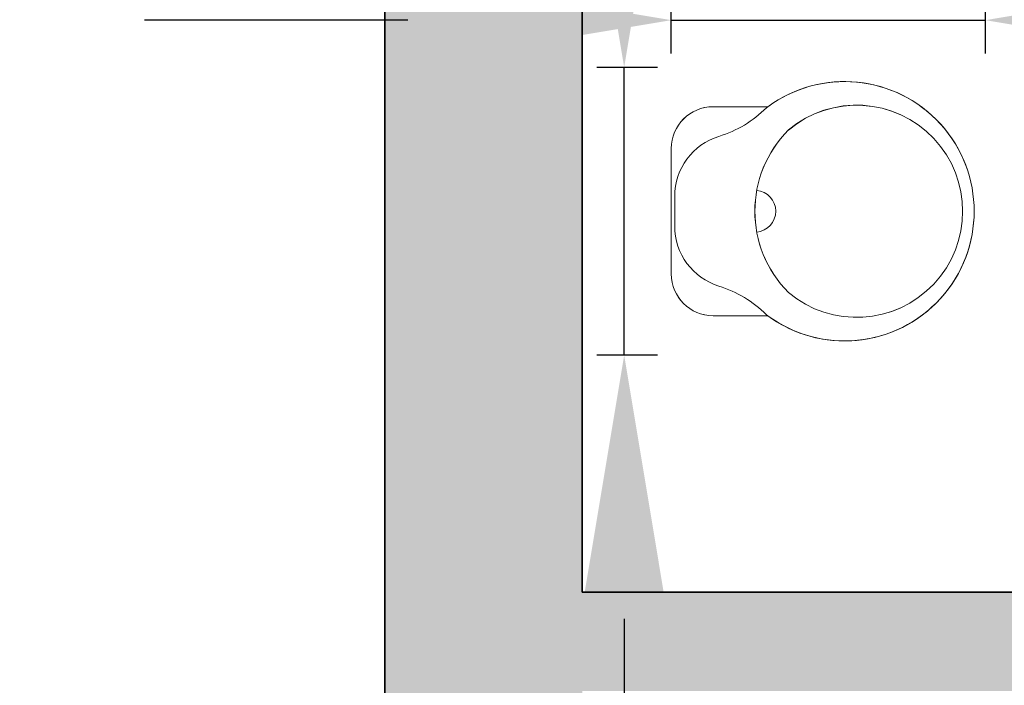
# Model space of a CAD drawing. Units: inches. Extents: x 2083 to 3317, y 1141 to 2115.
# Tile 15 of 256: x 2210 to 2255, y 1417 to 1447. Entities that reach past the tile are written whole.
import ezdxf

# ---------------------------------------------------------------- set-up
doc = ezdxf.new("R2010")
doc.units = ezdxf.units.IN
for name, color, linetype, lineweight in [('A-ANNO-DIMS', 2, 'Continuous', 18), ('A-FLOR-FIXT', 9, 'Continuous', 18), ('A-WALL', 7, 'Continuous', 35)]:
    doc.layers.add(name, color=color, linetype=linetype, lineweight=lineweight)
doc.layers.add('A-WALL-PATT', color=251, linetype='Continuous', lineweight=13, true_color=0x636466)
doc.styles.get("Standard").update_dxf_attribs({"font": 'arial.ttf'})
doc.dimstyles.new('ISO-25', dxfattribs={"dimtxt": 12, "dimasz": 12, "dimexe": 1.25, "dimexo": 0.625, "dimtad": 1, "dimlunit": 3, "dimtxsty": 'Standard', "dimcen": 2.5, "dimadec": 0, "dimazin": 0, "dimtfac": 1, "dimtmove": 0, "dimatfit": 3, "dimfxl": 1, "dimarcsym": 0})

# ---------------------------------------------------------------- blocks, each defined once
blk = doc.blocks.new('A$C6EF51710')
at = {"linetype": 'ByBlock'}
for p, q in [((0.0508, 0.2843), (0.1169, 0.2843)), ((0, 0.0811), (0, 0.2335)), ((0.0041, 0.1392), (0.0041, 0.1755)), ((0.1169, 0.0303), (0.0508, 0.0303))]:
    blk.add_line(p, q, dxfattribs=at)
for centre, radius, start, end in [((0.2107, 0.1573), 0.1576, 232.8984, 127.1016), ((0.0508, 0.2335), 0.0508, 90, 180), ((0.0168, 0.3818), 0.1397, 287.1046, 315), ((0.2254, 0.1573), 0.1289, 230.0084, 129.9916), ((0.2413, 0.1573), 0.1397, 135, 225), ((0.0803, 0.1755), 0.0762, 107.1046, 180), ((0.1016, 0.1573), 0.0254, 275.2159, 84.7841), ((0.0803, 0.1392), 0.0762, 180, 252.8954), ((0.0508, 0.0811), 0.0508, 180, 270), ((0.0168, -0.0672), 0.1397, 45, 72.8954)]:
    blk.add_arc(centre, radius, start, end, dxfattribs=at)
blk = doc.blocks.new('*D13')
at = {"layer": 'A-ANNO-DIMS', "color": 0, "lineweight": -2, "transparency": 16777216}
for p, q in [((2226.335, 1477.761), (2191.976, 1477.761)), ((2193.226, 1465.761), (2193.226, 1275.261)), ((2226.335, 1263.261), (2191.976, 1263.261))]:
    blk.add_line(p, q, dxfattribs=at)
at = {"layer": 'A-ANNO-DIMS', "color": 0, "transparency": 16777216}
for points in [[(2191.226, 1465.761), (2195.226, 1465.761), (2193.226, 1477.761)], [(2191.226, 1275.261), (2195.226, 1275.261), (2193.226, 1263.261)]]:
    blk.add_solid(points, dxfattribs=at)
at = {"layer": 'Defpoints', "color": 0, "transparency": 16777216}
for p in [(2226.96, 1477.761), (2193.226, 1263.261), (2226.96, 1263.261)]:
    blk.add_point(p, dxfattribs=at)
at = {"layer": 'A-ANNO-DIMS', "color": 0, "transparency": 16777216, "insert": (2186.474, 1370.511), "char_height": 12, "attachment_point": 5, "rotation": 90}
blk.add_mtext('17\'-10.5"', dxfattribs=at)
blk = doc.blocks.new('*D22')
at = {"layer": 'A-ANNO-DIMS', "color": 0, "lineweight": -2, "transparency": 16777216}
for p, q in [((2235.96, 1362.739), (2235.96, 1376.309)), ((2322.26, 1362.739), (2322.26, 1376.309)), ((2235.96, 1375.059), (2083.007, 1375.059)), ((2310.26, 1375.059), (2247.96, 1375.059))]:
    blk.add_line(p, q, dxfattribs=at)
at = {"layer": 'A-ANNO-DIMS', "color": 0, "transparency": 16777216}
for points in [[(2247.96, 1377.059), (2247.96, 1373.059), (2235.96, 1375.059)], [(2310.26, 1377.059), (2310.26, 1373.059), (2322.26, 1375.059)]]:
    blk.add_solid(points, dxfattribs=at)
at = {"layer": 'Defpoints', "color": 0, "transparency": 16777216}
for p in [(2235.96, 1375.059), (2235.96, 1362.114), (2322.26, 1362.114)]:
    blk.add_point(p, dxfattribs=at)
at = {"layer": 'A-ANNO-DIMS', "color": 0, "transparency": 16777216, "insert": (2153.483, 1381.889), "char_height": 12, "attachment_point": 5}
blk.add_mtext('BED 7\'-2 1/2" TYP.', dxfattribs=at)
blk = doc.blocks.new('*D30')
at = {"layer": 'A-ANNO-DIMS', "color": 0, "lineweight": -2, "transparency": 16777216}
for p, q in [((2240.018, 1445.274), (2240.018, 1448.046)), ((2254.329, 1445.274), (2254.329, 1448.046)), ((2228.018, 1446.796), (2216.018, 1446.796)), ((2240.018, 1446.796), (2254.329, 1446.796)), ((2266.329, 1446.796), (2413.765, 1446.796))]:
    blk.add_line(p, q, dxfattribs=at)
at = {"layer": 'A-ANNO-DIMS', "color": 0, "transparency": 16777216}
for points in [[(2228.018, 1448.796), (2228.018, 1444.796), (2240.018, 1446.796)], [(2266.329, 1448.796), (2266.329, 1444.796), (2254.329, 1446.796)]]:
    blk.add_solid(points, dxfattribs=at)
at = {"layer": 'Defpoints', "color": 0, "transparency": 16777216}
for p in [(2254.329, 1446.796), (2240.018, 1444.649), (2254.329, 1444.649)]:
    blk.add_point(p, dxfattribs=at)
at = {"layer": 'A-ANNO-DIMS', "color": 0, "transparency": 16777216, "insert": (2346.047, 1453.625), "char_height": 12, "attachment_point": 5}
blk.add_mtext('WC 1\'-2 1/2" TYP.', dxfattribs=at)
blk = doc.blocks.new('*D31')
at = {"layer": 'A-ANNO-DIMS', "color": 0, "lineweight": -2, "transparency": 16777216}
for p, q in [((2237.871, 1456.649), (2237.871, 1541.915)), ((2239.393, 1444.649), (2236.621, 1444.649)), ((2237.871, 1431.548), (2237.871, 1444.649)), ((2239.393, 1431.548), (2236.621, 1431.548)), ((2237.871, 1419.548), (2237.871, 1407.548))]:
    blk.add_line(p, q, dxfattribs=at)
at = {"layer": 'A-ANNO-DIMS', "color": 0, "transparency": 16777216}
for points in [[(2235.871, 1456.649), (2239.871, 1456.649), (2237.871, 1444.649)], [(2235.871, 1419.548), (2239.871, 1419.548), (2237.871, 1431.548)]]:
    blk.add_solid(points, dxfattribs=at)
at = {"layer": 'Defpoints', "color": 0, "transparency": 16777216}
for p in [(2237.871, 1444.649), (2240.018, 1444.649), (2240.018, 1431.548)]:
    blk.add_point(p, dxfattribs=at)
at = {"layer": 'A-ANNO-DIMS', "color": 0, "transparency": 16777216, "insert": (2231.217, 1505.282), "char_height": 12, "attachment_point": 5, "rotation": 90}
blk.add_mtext('1\'-1" TYP.', dxfattribs=at)

msp = doc.modelspace()

# ---------------------------------------------------------------- hatches: boundary and pattern name
at = {"layer": 'A-WALL-PATT'}
h = msp.add_hatch(color=256, dxfattribs=at)
h.dxf.hatch_style = 1
h.paths.add_polyline_path([(3126.96, 2020.761), (2748.96, 2020.761), (2604.96, 2020.761), (2226.96, 2020.761), (2226.96, 1702.761), (2466.96, 1702.761), (2466.96, 1582.761), (2418.96, 1582.761), (2418.96, 1477.761), (2226.96, 1477.761), (2226.96, 1263.261), (2544.96, 1263.261), (2544.96, 1411.761), (2604.96, 1411.761), (2685.96, 1411.761), (2685.96, 1420.761), (2604.96, 1420.761), (2604.96, 1573.761), (2604.96, 1702.761), (2604.96, 2011.761), (2748.96, 2011.761), (2748.96, 1702.761), (2862.96, 1702.761), (2862.96, 1621.761), (2871.96, 1621.761), (2871.96, 1702.761), (2883.96, 1702.761), (2883.96, 1706.939, -0.026459), (2883.96, 1711.761), (2757.96, 1711.761), (2757.96, 1807.761), (2787.96, 1807.761), (2787.96, 1812.261), (2757.96, 1812.261), (2757.96, 2011.761), (2877.96, 2011.761), (2877.96, 1812.261), (2847.96, 1812.261), (2847.96, 1807.761), (2889.836, 1807.761), (2889.836, 1812.261), (2882.46, 1812.261), (2882.46, 2011.761), (3117.96, 2011.761), (3117.96, 1812.261), (2937.836, 1812.261), (2937.836, 1807.761), (2995.71, 1807.761), (2995.71, 1796.118), (3000.21, 1796.118), (3000.21, 1807.761), (3117.96, 1807.761), (3117.96, 1711.761), (3000.21, 1711.761), (3000.21, 1760.118), (2998.573, 1760.118, -0.020711), (2995.71, 1760.118), (2995.71, 1711.761), (2931.96, 1711.761), (2931.96, 1702.761), (3126.96, 1702.761)])
h.paths.add_polyline_path([(2471.46, 2011.761), (2471.46, 1810.011), (2462.717, 1810.011), (2462.717, 1805.511), (2505.96, 1805.511), (2505.96, 1810.011), (2475.96, 1810.011), (2475.96, 2011.761), (2595.96, 2011.761), (2595.96, 1810.011), (2565.96, 1810.011), (2565.96, 1805.511), (2595.96, 1805.511), (2595.96, 1711.761), (2235.96, 1711.761), (2235.96, 1805.511), (2353.71, 1805.511), (2353.71, 1796.054), (2358.21, 1796.054), (2358.21, 1805.511), (2414.717, 1805.511), (2414.717, 1810.011), (2235.96, 1810.011), (2235.96, 2011.761)], flags=16)
h.paths.add_polyline_path([(2270.205, 1994.61), (2270.205, 1970.61), (2246.205, 1970.61), (2246.205, 1994.61)], flags=0)
edge = h.paths.add_edge_path(flags=0)
edge.add_ellipse((2332.027, 1899.798), major_axis=(-3.043, 3.043), ratio=0.168252, start_angle=-161.3322, end_angle=-156.3071, ccw=False)
edge.add_ellipse((2333.082, 1898.744), major_axis=(-1.055, 1.055), ratio=0.453532, start_angle=-123.371, end_angle=-94.1591)
edge = h.paths.add_edge_path(flags=0)
edge.add_ellipse((2332.027, 1968.876), major_axis=(3.043, 3.043), ratio=0.168252, start_angle=18.6678, end_angle=23.6929)
edge.add_spline(control_points=[(2332.926, 1970.691), (2332.227, 1970.336), (2330.894, 1969.659), (2328.413, 1970.932), (2327.204, 1967.749), (2324.71, 1969.956), (2322.533, 1967.012), (2320.013, 1971.296), (2317.68, 1968.158), (2316.041, 1967.102), (2315.427, 1966.81)], knot_values=[0, 0, 0, 0, 2.267059, 4.324559, 6.685584, 8.878641, 11.121502, 14.300359, 17.755284, 19.732645, 19.732645, 19.732645, 19.732645], degree=3, periodic=0)
edge.add_ellipse((2332.027, 1968.876), major_axis=(3.043, 3.043), ratio=0.168252, start_angle=18.6678, end_angle=23.6929, ccw=False)
edge.add_ellipse((2333.082, 1969.931), major_axis=(1.055, 1.055), ratio=0.453532, start_angle=56.629, end_angle=85.8409, ccw=False)
edge = h.paths.add_edge_path(flags=0)
edge.add_spline(control_points=[(2296.428, 1967.988), (2293.628, 1965.336), (2287.704, 1959.727), (2299.744, 1949.996), (2294.533, 1935.669), (2290.573, 1920.604), (2293.394, 1909.974), (2296.185, 1904.967)], knot_values=[0.099185, 0.099185, 0.099185, 0.099185, 0.345301, 0.619822, 0.982653, 1.386093, 1.810555, 1.810555, 1.810555, 1.810555], degree=3, periodic=0)
edge.add_spline(control_points=[(2296.185, 1904.967), (2297.384, 1902.619), (2298.001, 1901.949), (2298.553, 1901.468)], knot_values=[0.006246, 0.006246, 0.006246, 0.006246, 0.055476, 0.055476, 0.055476, 0.055476], degree=3, periodic=0)
edge.add_spline(control_points=[(2298.553, 1901.468), (2297.259, 1900.923), (2295.225, 1900.232), (2293.06, 1900.614), (2292.101, 1900.788), (2292.09, 1900.791)], knot_values=[0.312835, 0.312835, 0.312835, 0.312835, 0.40178, 0.474987, 0.475903, 0.475903, 0.475903, 0.475903], degree=3, periodic=0)
edge.add_arc((2292.794, 1904.664), 3.937, 215.4209, 259.6982, ccw=False)
edge.add_spline(control_points=[(2289.585, 1902.382), (2289.477, 1902.535), (2289.368, 1902.688), (2289.261, 1902.841)], knot_values=[0.102872, 0.102872, 0.102872, 0.102872, 0.116896, 0.116896, 0.116896, 0.116896], degree=3, periodic=0)
edge.add_spline(control_points=[(2289.261, 1902.841), (2288.687, 1902.55), (2287.64, 1902.02), (2285.881, 1901.874), (2283.853, 1901.504), (2281.72, 1899.711), (2278.467, 1899.493), (2276.157, 1901.883), (2272.259, 1899.804), (2267.778, 1901.843), (2262.244, 1900.184), (2257.415, 1901.782), (2254.318, 1900.726), (2253.178, 1900.337)], knot_values=[0, 0, 0, 0, 1.907977, 3.477176, 5.261074, 7.972851, 11.680248, 13.717921, 16.939592, 22.789562, 27.502503, 33.595215, 37.145618, 37.145618, 37.145618, 37.145618], degree=3, periodic=0)
edge.add_line((2253.178, 1900.337), (2250.244, 1902.841))
edge.add_line((2250.244, 1902.841), (2250.244, 1965.833))
edge.add_line((2250.244, 1965.833), (2253.178, 1968.337))
edge.add_spline(control_points=[(2253.178, 1968.337), (2254.318, 1967.948), (2257.415, 1966.892), (2262.244, 1968.49), (2267.778, 1966.831), (2271.527, 1968.537), (2273.876, 1967.828), (2274.207, 1967.728)], knot_values=[0, 0, 0, 0, 0.09018, 0.244935, 0.364644, 0.513233, 0.537855, 0.537855, 0.537855, 0.537855], degree=3, periodic=0)
edge.add_arc((2274.353, 1963.793), 3.937, 72.0511, 92.1279, ccw=False)
edge.add_arc((2281.297, 1985.23), 18.596, 252.0511, 288.5657)
edge.add_arc((2292.317, 1956.029), 12.646, 71.0268, 113.7782, ccw=False)
edge = h.paths.add_edge_path(flags=0)
edge.add_spline(control_points=[(2274.899, 1951.856), (2275.066, 1951.617), (2275.233, 1951.377), (2275.398, 1951.136)], knot_values=[1.409916, 1.409916, 1.409916, 1.409916, 1.43159, 1.43159, 1.43159, 1.43159], degree=3, periodic=0)
edge.add_spline(control_points=[(2275.398, 1951.136), (2275.792, 1950.562), (2276.179, 1949.984), (2276.546, 1949.397)], knot_values=[1.358238, 1.358238, 1.358238, 1.358238, 1.409916, 1.409916, 1.409916, 1.409916], degree=3, periodic=0)
edge.add_line((2276.546, 1949.397), (2277.437, 1947.862))
edge.add_spline(control_points=[(2277.437, 1947.862), (2276.304, 1945.673), (2274.64, 1942.427), (2274.632, 1938.094), (2272.799, 1930.852), (2274.356, 1943.897), (2275.948, 1947.923), (2276.546, 1949.397)], knot_values=[0.005632, 0.005632, 0.005632, 0.005632, 0.186014, 0.266002, 0.357087, 0.59639, 0.739732, 0.739732, 0.739732, 0.739732], degree=3, periodic=0)
edge.add_spline(control_points=[(2276.546, 1949.397), (2276.179, 1949.984), (2275.792, 1950.562), (2275.398, 1951.136)], knot_values=[1.358238, 1.358238, 1.358238, 1.358238, 1.409916, 1.409916, 1.409916, 1.409916], degree=3, periodic=0)
edge.add_spline(control_points=[(2275.398, 1951.136), (2274.943, 1950.08), (2274.208, 1948.025), (2273.935, 1944.851), (2272.469, 1937.627), (2273.466, 1945.696), (2274.701, 1951.059), (2274.899, 1951.856)], knot_values=[0.104364, 0.104364, 0.104364, 0.104364, 0.189636, 0.269624, 0.36071, 0.600013, 0.644622, 0.644622, 0.644622, 0.644622], degree=3, periodic=0)
h.paths.add_polyline_path([(2269.168, 1963.128, -0.357527), (2268.171, 1960.976, -0.092561), (2268.171, 1939.436, -0.357527), (2269.168, 1937.285, -0.357527), (2267.016, 1938.282, -0.164785), (2254.686, 1938.282, -0.357527), (2252.534, 1937.285, -0.357527), (2253.531, 1939.436, -0.092561), (2253.531, 1960.976, -0.357527), (2252.534, 1963.128, -0.357527), (2254.686, 1962.131, -0.164785), (2267.016, 1962.131, -0.357527)], flags=0)
h.paths.add_polyline_path([(2248.874, 1967.802), (2248.874, 1957.028), (2249.458, 1957.028), (2249.458, 1911.647), (2248.874, 1911.647), (2248.874, 1900.873), (2246.512, 1900.873, 0.197327), (2244.15, 1902.457), (2244.15, 1966.218, 0.197327), (2246.512, 1967.802)], flags=0)
h.paths.add_polyline_path([(2269.168, 1931.389, -0.357527), (2268.171, 1929.238, -0.092561), (2268.171, 1907.698, -0.357527), (2269.168, 1905.547, -0.357527), (2267.016, 1906.544, -0.164785), (2254.686, 1906.544, -0.357527), (2252.534, 1905.547, -0.357527), (2253.531, 1907.698, -0.092561), (2253.531, 1929.238, -0.357527), (2252.534, 1931.389, -0.357527), (2254.686, 1930.392, -0.164785), (2267.016, 1930.392, -0.357527)], flags=0)
edge = h.paths.add_edge_path(flags=0)
edge.add_spline(control_points=[(2276.197, 1906.724), (2276.168, 1909.029), (2276.114, 1913.372), (2270.598, 1924.925), (2273.905, 1919.013), (2275.922, 1916.262), (2275.475, 1912.402), (2277.258, 1910.381), (2276.696, 1908.225), (2276.646, 1906.813), (2276.618, 1906.008)], knot_values=[0, 0, 0, 0, 8.61026, 16.221274, 18.843057, 23.804898, 27.440828, 29.356102, 31.203478, 33.650687, 33.650687, 33.650687, 33.650687], degree=3, periodic=0)
edge.add_spline(control_points=[(2276.618, 1906.008), (2276.623, 1905.624), (2276.498, 1904.629), (2275.442, 1903.855), (2274.937, 1903.08), (2274.859, 1902.841)], knot_values=[0.156488, 0.156488, 0.156488, 0.156488, 0.184398, 0.231376, 0.250598, 0.250598, 0.250598, 0.250598], degree=3, periodic=0)
edge.add_line((2274.859, 1902.841), (2276.506, 1902.841))
edge.add_spline(control_points=[(2276.506, 1902.841), (2276.788, 1903.085), (2277.665, 1904.125), (2278.25, 1904.341), (2277.654, 1908.527), (2278.156, 1906.228), (2278.1, 1905.286), (2278.847, 1904.069), (2277.857, 1903.415), (2277.874, 1902.991), (2277.904, 1902.841)], knot_values=[0.059574, 0.059574, 0.059574, 0.059574, 0.080753, 0.103741, 0.16972, 0.176036, 0.207137, 0.240474, 0.262341, 0.27366, 0.27366, 0.27366, 0.27366], degree=3, periodic=0)
edge.add_line((2277.904, 1902.841), (2280.03, 1902.841))
edge.add_spline(control_points=[(2280.03, 1902.841), (2279.888, 1903.088), (2279.499, 1903.982), (2280.152, 1905.939), (2278.104, 1909.658), (2279.762, 1907.185), (2280.328, 1904.875), (2280.485, 1903.49), (2281.463, 1903.249), (2281.758, 1902.936), (2281.834, 1902.841)], knot_values=[0.013856, 0.013856, 0.013856, 0.013856, 0.034874, 0.088867, 0.107879, 0.126738, 0.158714, 0.193757, 0.217487, 0.226722, 0.226722, 0.226722, 0.226722], degree=3, periodic=0)
edge.add_spline(control_points=[(2281.834, 1902.841), (2281.788, 1902.827), (2281.647, 1902.783), (2281.396, 1902.859), (2281.088, 1902.985), (2280.721, 1903.061), (2280.333, 1903.026), (2280.125, 1902.899), (2280.03, 1902.841)], knot_values=[0, 0, 0, 0, 0.14413, 0.435517, 0.749276, 1.153046, 1.548371, 1.878348, 1.878348, 1.878348, 1.878348], degree=3, periodic=0)
edge.add_line((2280.03, 1902.841), (2277.904, 1902.841))
edge.add_spline(control_points=[(2277.904, 1902.841), (2277.893, 1902.796), (2277.865, 1902.68), (2277.607, 1902.687), (2277.274, 1902.801), (2276.838, 1902.62), (2276.584, 1902.789), (2276.506, 1902.841)], knot_values=[0, 0, 0, 0, 0.127189, 0.326199, 0.628009, 1.24357, 1.515331, 1.515331, 1.515331, 1.515331], degree=3, periodic=0)
edge.add_line((2276.506, 1902.841), (2274.859, 1902.841))
edge.add_spline(control_points=[(2274.859, 1902.841), (2274.814, 1902.899), (2274.725, 1903.013), (2274.493, 1903.119), (2274.244, 1902.961), (2273.937, 1903.185), (2273.614, 1902.983), (2273.408, 1902.883), (2273.322, 1902.841)], knot_values=[0, 0, 0, 0, 0.21843, 0.436957, 0.687977, 0.990379, 1.398396, 1.69185, 1.69185, 1.69185, 1.69185], degree=3, periodic=0)
edge.add_spline(control_points=[(2273.322, 1902.841), (2273.617, 1903.446), (2274.274, 1904.538), (2276.027, 1904.574), (2276.207, 1906.584), (2276.197, 1906.724)], knot_values=[0.012227, 0.012227, 0.012227, 0.012227, 0.059472, 0.106218, 0.134458, 0.134458, 0.134458, 0.134458], degree=3, periodic=0)
h.paths.add_polyline_path([(2270.776, 1897.79), (2270.776, 1873.79), (2246.776, 1873.79), (2246.776, 1897.79)], flags=0)
h.paths.add_polyline_path([(2353.71, 1760.005), (2353.71, 1760.054), (2358.21, 1760.054, -0.033729)], flags=0)
h.paths.add_polyline_path([(2321.819, 1737.529), (2341.995, 1737.529, -0.414214), (2343.203, 1736.321), (2343.203, 1721.021, -0.414214), (2341.995, 1719.813), (2321.819, 1719.813, -0.414214), (2320.611, 1721.021), (2320.611, 1736.321, -0.414214)], flags=0)
h.paths.add_polyline_path([(2324.235, 1736.321), (2339.579, 1736.321, -0.414214), (2341.995, 1733.905), (2341.995, 1725.45, -0.414214), (2339.579, 1723.034), (2333.681, 1723.034), (2333.845, 1722.045, -0.870646), (2335.425, 1721.826, -0.767327), (2333.923, 1721.423), (2331.291, 1721.423, -0.767327), (2329.788, 1721.826, -0.870646), (2331.368, 1722.045), (2331.533, 1723.034), (2324.235, 1723.034, -0.414214), (2321.819, 1725.45), (2321.819, 1733.905, -0.414214)], flags=0)
h.paths.add_polyline_path([(2570.484, 1928.615), (2589.684, 1928.615), (2590.169, 1928.615), (2590.169, 1904.993), (2570.484, 1904.993)], flags=0)
h.paths.add_polyline_path([(2574.447, 1927.264, -1), (2572.829, 1927.264, -1)], flags=0)
h.paths.add_polyline_path([(2573.09, 1926.941), (2573.925, 1927.776), (2574.148, 1927.553), (2573.313, 1926.718)], flags=0)
h.paths.add_polyline_path([(2578.779, 1919.73, -1), (2571.592, 1919.73, -1)], flags=0)
h.paths.add_polyline_path([(2578.385, 1919.73, -1), (2571.985, 1919.73, -1)], flags=0)
h.paths.add_polyline_path([(2331.596, 1729.476, -1), (2333.618, 1729.476, -1)], flags=0)
h.paths.add_polyline_path([(2578.034, 1927.264, -1), (2576.416, 1927.264, -1)], flags=0)
h.paths.add_polyline_path([(2576.689, 1927.531), (2576.912, 1927.754), (2577.747, 1926.919), (2577.524, 1926.696)], flags=0)
h.paths.add_polyline_path([(2578.139, 1909.86, -1), (2572.232, 1909.86, -1)], flags=0)
h.paths.add_polyline_path([(2577.745, 1909.86, -1), (2572.625, 1909.86, -1)], flags=0)
h.paths.add_polyline_path([(2583.798, 1927.264, -1), (2582.179, 1927.264, -1)], flags=0)
h.paths.add_polyline_path([(2582.719, 1927.754), (2583.554, 1926.919), (2583.331, 1926.696), (2582.496, 1927.531)], flags=0)
h.paths.add_polyline_path([(2582.496, 1927.531), (2582.719, 1927.754), (2583.554, 1926.919), (2583.331, 1926.696)], flags=0)
h.paths.add_polyline_path([(2587.739, 1920.53, -1), (2581.832, 1920.53, -1)], flags=0)
h.paths.add_polyline_path([(2587.345, 1920.53, -1), (2582.225, 1920.53, -1)], flags=0)
h.paths.add_polyline_path([(2587.385, 1927.264, -1), (2585.766, 1927.264, -1)], flags=0)
h.paths.add_polyline_path([(2586.082, 1926.98), (2586.917, 1927.815), (2587.14, 1927.593), (2586.305, 1926.758)], flags=0)
h.paths.add_polyline_path([(2588.379, 1910.66, -1), (2581.192, 1910.66, -1)], flags=0)
h.paths.add_polyline_path([(2587.985, 1910.66, -1), (2581.585, 1910.66, -1)], flags=0)
h.paths.add_polyline_path([(2417.168, 1729.478), (2437.344, 1729.478, -0.414214), (2438.552, 1728.27), (2438.552, 1712.969, -0.414214), (2437.344, 1711.761), (2417.168, 1711.761, -0.414214), (2415.96, 1712.969), (2415.96, 1728.27, -0.414214)], flags=0)
h.paths.add_polyline_path([(2419.584, 1728.27), (2434.928, 1728.27, -0.414214), (2437.344, 1725.854), (2437.344, 1717.398, -0.414214), (2434.928, 1714.983), (2429.029, 1714.983), (2429.194, 1713.994, -0.870646), (2430.774, 1713.775, -0.767327), (2429.271, 1713.372), (2426.64, 1713.372, -0.767327), (2425.137, 1713.775, -0.870646), (2426.717, 1713.994), (2426.882, 1714.983), (2419.584, 1714.983, -0.414214), (2417.168, 1717.398), (2417.168, 1725.854, -0.414214)], flags=0)
h.paths.add_polyline_path([(2419.584, 1728.27), (2434.928, 1728.27, -0.414214), (2437.344, 1725.854), (2437.344, 1717.398, -0.414214), (2434.928, 1714.983), (2429.029, 1714.983), (2428.358, 1719.009), (2427.553, 1719.009), (2426.882, 1714.983), (2419.584, 1714.983, -0.414214), (2417.168, 1717.398), (2417.168, 1725.854, -0.414214)], flags=0)
h.paths.add_polyline_path([(2426.944, 1721.425, -1), (2428.967, 1721.425, -1)], flags=0)
h.paths.add_polyline_path([(2475.96, 1702.761), (2595.96, 1702.761), (2595.96, 1582.761), (2475.96, 1582.761)], flags=16)
h.paths.add_polyline_path([(2427.96, 1573.761), (2595.96, 1573.761), (2595.96, 1468.761), (2595.96, 1420.761), (2384.46, 1420.761), (2384.46, 1468.761), (2427.96, 1468.761)], flags=16)
h.paths.add_polyline_path([(2379.96, 1468.761), (2379.96, 1420.761), (2235.96, 1420.761), (2235.96, 1468.761)], flags=16)
h.paths.add_polyline_path([(2317.816, 1466.696), (2337.992, 1466.696, -0.414214), (2339.2, 1465.488), (2339.2, 1450.187, -0.414214), (2337.992, 1448.979), (2317.816, 1448.979, -0.414214), (2316.608, 1450.187), (2316.608, 1465.488, -0.414214)], flags=0)
h.paths.add_polyline_path([(2320.232, 1465.488), (2335.576, 1465.488, -0.414214), (2337.992, 1463.072), (2337.992, 1454.616, -0.414214), (2335.576, 1452.2), (2329.677, 1452.2), (2329.842, 1451.212, -0.870646), (2331.422, 1450.992, -0.767327), (2329.92, 1450.59), (2327.288, 1450.59, -0.767327), (2325.785, 1450.992, -0.870646), (2327.365, 1451.212), (2327.53, 1452.2), (2320.232, 1452.2, -0.414214), (2317.816, 1454.616), (2317.816, 1463.072, -0.414214)], flags=0)
h.paths.add_polyline_path([(2320.232, 1465.488), (2335.576, 1465.488, -0.414214), (2337.992, 1463.072), (2337.992, 1454.616, -0.414214), (2335.576, 1452.2), (2329.677, 1452.2), (2329.006, 1456.227), (2328.201, 1456.227), (2327.53, 1452.2), (2320.232, 1452.2, -0.414214), (2317.816, 1454.616), (2317.816, 1463.072, -0.414214)], flags=0)
h.paths.add_polyline_path([(2327.593, 1458.643, -1), (2329.615, 1458.643, -1)], flags=0)
h.paths.add_polyline_path([(2244.412, 1433.34), (2241.921, 1433.34, -0.414214), (2240.018, 1435.244), (2240.018, 1440.953, -0.414211), (2241.921, 1442.856), (2244.412, 1442.856, -1.976472)], flags=0)
h.paths.add_polyline_path([(2245.357, 1434.398, -0.414214), (2245.357, 1441.799, -2.144098)], flags=0)
h.paths.add_polyline_path([(2535.96, 1416.261), (2535.96, 1272.261), (2235.96, 1272.261), (2235.96, 1416.261)], flags=16)
h.paths.add_polyline_path([(2260.12, 1384.293), (2260.12, 1362.039), (2237.865, 1362.039), (2237.865, 1384.293)], flags=0)
edge = h.paths.add_edge_path(flags=0)
edge.add_line((2318.252, 1362.093), (2318.146, 1362.001))
edge.add_ellipse((2317.445, 1360.431), major_axis=(2.822, 2.822), ratio=0.168252, start_angle=18.6678, end_angle=20.9481, ccw=False)
edge.add_ellipse((2318.423, 1361.409), major_axis=(0.978, 0.978), ratio=0.453532, start_angle=56.629, end_angle=70.2262, ccw=False)
edge = h.paths.add_edge_path(flags=0)
edge.add_line((2319.107, 1295.571), (2319.015, 1295.677))
edge.add_ellipse((2317.445, 1296.378), major_axis=(-2.822, 2.822), ratio=0.168252, start_angle=-161.3322, end_angle=-159.0519, ccw=False)
edge.add_ellipse((2318.423, 1295.4), major_axis=(-0.978, 0.978), ratio=0.453532, start_angle=-123.371, end_angle=-109.7738)
edge = h.paths.add_edge_path(flags=0)
edge.add_spline(control_points=[(2284.21, 1301.17), (2284.581, 1300.445), (2284.891, 1299.892), (2285.16, 1299.461)], knot_values=[0.039066, 0.039066, 0.039066, 0.039066, 0.055476, 0.055476, 0.055476, 0.055476], degree=3, periodic=0)
edge.add_line((2285.16, 1299.461), (2284.21, 1301.17))
edge = h.paths.add_edge_path(flags=0)
edge.add_line((2280.412, 1297.298), (2283.37, 1297.036))
edge.add_line((2283.37, 1297.036), (2286.406, 1297.926))
edge.add_spline(control_points=[(2286.406, 1297.926), (2285.305, 1297.463), (2284.345, 1297.129), (2283.37, 1297.036)], knot_values=[0.394369, 0.394369, 0.394369, 0.394369, 0.475903, 0.475903, 0.475903, 0.475903], degree=3, periodic=0)
edge.add_spline(control_points=[(2283.37, 1297.036), (2283.281, 1297.028), (2282.316, 1296.957), (2281.313, 1297.134), (2280.423, 1297.296), (2280.412, 1297.298)], knot_values=[0.312835, 0.312835, 0.312835, 0.312835, 0.320246, 0.393453, 0.394369, 0.394369, 0.394369, 0.394369], degree=3, periodic=0)
edge = h.paths.add_edge_path(flags=0)
edge.add_line((2284.436, 1359.607), (2280.446, 1355.328))
edge.add_line((2280.446, 1355.328), (2279.58, 1351.018))
edge.add_line((2279.58, 1351.018), (2282.413, 1346.58))
edge.add_spline(control_points=[(2282.413, 1346.58), (2283.153, 1345.589), (2284.253, 1344.029), (2284.801, 1342.387), (2284.935, 1341.806)], knot_values=[1.240098, 1.240098, 1.240098, 1.240098, 1.332892, 1.382712, 1.382712, 1.382712, 1.382712], degree=3, periodic=0)
edge.add_spline(control_points=[(2284.935, 1341.806), (2285.319, 1340.141), (2285.233, 1338.409), (2284.91, 1336.654)], knot_values=[1.097484, 1.097484, 1.097484, 1.097484, 1.240098, 1.240098, 1.240098, 1.240098], degree=3, periodic=0)
edge.add_spline(control_points=[(2284.91, 1336.654), (2284.587, 1334.899), (2284.027, 1333.12), (2283.463, 1331.361)], knot_values=[0.95487, 0.95487, 0.95487, 0.95487, 1.097484, 1.097484, 1.097484, 1.097484], degree=3, periodic=0)
edge.add_line((2283.463, 1331.361), (2281.89, 1326.153))
edge.add_line((2281.89, 1326.153), (2280.756, 1321.056))
edge.add_line((2280.756, 1321.056), (2280.299, 1316.002))
edge.add_line((2280.299, 1316.002), (2280.716, 1310.95))
edge.add_line((2280.716, 1310.95), (2282.028, 1305.972))
edge.add_line((2282.028, 1305.972), (2284.21, 1301.17))
edge.add_spline(control_points=[(2284.21, 1301.17), (2283.341, 1302.73), (2282.612, 1304.336), (2282.028, 1305.972)], knot_values=[0.099185, 0.099185, 0.099185, 0.099185, 0.241799, 0.241799, 0.241799, 0.241799], degree=3, periodic=0)
edge.add_spline(control_points=[(2282.028, 1305.972), (2281.444, 1307.608), (2281.005, 1309.273), (2280.716, 1310.95)], knot_values=[0.241799, 0.241799, 0.241799, 0.241799, 0.384413, 0.384413, 0.384413, 0.384413], degree=3, periodic=0)
edge.add_spline(control_points=[(2280.716, 1310.95), (2280.433, 1312.588), (2280.289, 1314.277), (2280.299, 1315.962), (2280.299, 1316.002)], knot_values=[0.384413, 0.384413, 0.384413, 0.384413, 0.523647, 0.527028, 0.527028, 0.527028, 0.527028], degree=3, periodic=0)
edge.add_spline(control_points=[(2280.299, 1316.002), (2280.312, 1317.687), (2280.478, 1319.368), (2280.756, 1321.056)], knot_values=[0.527028, 0.527028, 0.527028, 0.527028, 0.669642, 0.669642, 0.669642, 0.669642], degree=3, periodic=0)
edge.add_spline(control_points=[(2280.756, 1321.056), (2281.035, 1322.744), (2281.426, 1324.44), (2281.89, 1326.153)], knot_values=[0.669642, 0.669642, 0.669642, 0.669642, 0.812256, 0.812256, 0.812256, 0.812256], degree=3, periodic=0)
edge.add_spline(control_points=[(2281.89, 1326.153), (2282.264, 1327.533), (2282.788, 1329.262), (2283.353, 1331.018), (2283.463, 1331.361)], knot_values=[0.812256, 0.812256, 0.812256, 0.812256, 0.927087, 0.95487, 0.95487, 0.95487, 0.95487], degree=3, periodic=0)
edge.add_line((2283.463, 1331.361), (2284.91, 1336.654))
edge.add_line((2284.91, 1336.654), (2284.935, 1341.806))
edge.add_line((2284.935, 1341.806), (2282.413, 1346.58))
edge.add_spline(control_points=[(2282.413, 1346.58), (2281.275, 1348.104), (2280.078, 1349.57), (2279.58, 1351.018)], knot_values=[1.382712, 1.382712, 1.382712, 1.382712, 1.525326, 1.525326, 1.525326, 1.525326], degree=3, periodic=0)
edge.add_spline(control_points=[(2279.58, 1351.018), (2279.443, 1351.415), (2279.136, 1352.857), (2279.735, 1354.29), (2280.446, 1355.328)], knot_values=[1.525326, 1.525326, 1.525326, 1.525326, 1.564439, 1.667941, 1.667941, 1.667941, 1.667941], degree=3, periodic=0)
edge.add_spline(control_points=[(2280.446, 1355.328), (2281.426, 1356.758), (2282.931, 1358.183), (2284.436, 1359.607)], knot_values=[1.667941, 1.667941, 1.667941, 1.667941, 1.810555, 1.810555, 1.810555, 1.810555], degree=3, periodic=0)
edge.add_arc((2280.623, 1348.518), 11.726, 71.0268, 113.7782)
edge.add_arc((2270.405, 1375.595), 17.244, 252.0511, 288.5657, ccw=False)
edge.add_arc((2263.966, 1355.718), 3.651, 72.0511, 92.1279)
edge.add_arc((2263.966, 1355.718), 3.651, 92.1279, 177.9851)
edge.add_spline(control_points=[(2260.318, 1355.846), (2260.26, 1354.221), (2260.551, 1350.187), (2262.999, 1346.766), (2264.473, 1344.649)], knot_values=[1.43159, 1.43159, 1.43159, 1.43159, 1.564144, 1.770695, 1.770695, 1.770695, 1.770695], degree=3, periodic=0)
edge.add_line((2264.473, 1344.649), (2264.936, 1343.983))
edge.add_spline(control_points=[(2263.801, 1340.248), (2263.843, 1340.514), (2264.067, 1341.756), (2264.513, 1343.002), (2264.935, 1343.981)], knot_values=[0.53657, 0.53657, 0.53657, 0.53657, 0.559349, 0.644622, 0.644622, 0.644622, 0.644622], degree=3, periodic=0)
edge.add_spline(control_points=[(2264.935, 1343.981), (2265.118, 1343.715), (2265.299, 1343.448), (2265.477, 1343.179)], knot_values=[1.384077, 1.384077, 1.384077, 1.384077, 1.409916, 1.409916, 1.409916, 1.409916], degree=3, periodic=0)
edge.add_spline(control_points=[(2265.477, 1343.179), (2265.655, 1342.911), (2265.829, 1342.641), (2265.999, 1342.369)], knot_values=[1.358238, 1.358238, 1.358238, 1.358238, 1.384077, 1.384077, 1.384077, 1.384077], degree=3, periodic=0)
edge.add_line((2265.999, 1342.369), (2266.826, 1340.946))
edge.add_spline(control_points=[(2266.826, 1340.946), (2268.894, 1337.09), (2271.398, 1325.843), (2270.516, 1310.569), (2275.919, 1301.861), (2277.79, 1299.199)], knot_values=[0.116896, 0.116896, 0.116896, 0.116896, 0.472987, 1.050969, 1.313793, 1.313793, 1.313793, 1.313793], degree=3, periodic=0)
edge.add_spline(control_points=[(2277.79, 1299.199), (2277.839, 1299.128), (2277.889, 1299.057), (2277.94, 1298.987)], knot_values=[0.109884, 0.109884, 0.109884, 0.109884, 0.116896, 0.116896, 0.116896, 0.116896], degree=3, periodic=0)
edge.add_line((2277.94, 1298.987), (2277.789, 1299.199))
edge.add_spline(control_points=[(2277.789, 1299.199), (2277.257, 1298.929), (2276.286, 1298.438), (2275.039, 1298.334), (2274.383, 1298.239), (2274.215, 1298.209)], knot_values=[33.12187, 33.12187, 33.12187, 33.12187, 35.029056, 36.598255, 37.144827, 37.144827, 37.144827, 37.144827], degree=3, periodic=0)
edge.add_line((2274.215, 1298.209), (2273.073, 1297.893))
edge.add_spline(control_points=[(2273.073, 1297.893), (2272.323, 1297.58), (2271.039, 1296.511), (2269.248, 1296.226), (2268.423, 1296.375)], knot_values=[26.532584, 26.532584, 26.532584, 26.532584, 29.198919, 31.839101, 31.839101, 31.839101, 31.839101], degree=3, periodic=0)
edge.add_line((2268.423, 1296.375), (2263.879, 1297.458))
edge.add_spline(control_points=[(2263.879, 1297.458), (2263.556, 1297.359), (2261.86, 1296.839), (2260.239, 1297.282), (2258.933, 1297.516)], knot_values=[15.919551, 15.919551, 15.919551, 15.919551, 16.939592, 21.226067, 21.226067, 21.226067, 21.226067], degree=3, periodic=0)
edge.add_line((2258.933, 1297.516), (2254.055, 1297.329))
edge.add_spline(control_points=[(2254.055, 1297.329), (2253.756, 1297.296), (2252.114, 1297.165), (2250.462, 1297.544), (2249.13, 1297.668)], knot_values=[5.306517, 5.306517, 5.306517, 5.306517, 6.276435, 10.613034, 10.613034, 10.613034, 10.613034], degree=3, periodic=0)
edge.add_line((2249.13, 1297.668), (2244.332, 1296.878))
edge.add_line((2244.332, 1296.878), (2241.611, 1299.199))
edge.add_line((2241.611, 1299.199), (2241.611, 1357.609))
edge.add_line((2241.611, 1357.609), (2244.332, 1359.931))
edge.add_line((2244.332, 1359.931), (2252.729, 1359.543))
edge.add_spline(control_points=[(2252.729, 1359.543), (2252.871, 1359.546), (2253.306, 1359.548), (2253.74, 1359.514), (2254.032, 1359.482)], knot_values=[0.233291, 0.233291, 0.233291, 0.233291, 0.244935, 0.268927, 0.268927, 0.268927, 0.268927], degree=3, periodic=0)
edge.add_line((2254.032, 1359.482), (2259.587, 1359.416))
edge.add_spline(control_points=[(2259.587, 1359.416), (2260.677, 1359.629), (2262.073, 1359.897), (2263.524, 1359.459), (2263.83, 1359.366)], knot_values=[0.422516, 0.422516, 0.422516, 0.422516, 0.513233, 0.537855, 0.537855, 0.537855, 0.537855], degree=3, periodic=0)
edge.add_arc((2263.966, 1355.718), 3.651, 72.0511, 92.1279, ccw=False)
edge.add_arc((2270.405, 1375.595), 17.244, 252.0511, 288.5657)
edge.add_arc((2280.623, 1348.518), 11.726, 71.0268, 113.7782, ccw=False)
h.paths.add_polyline_path([(2240.341, 1359.435), (2240.341, 1349.444), (2240.882, 1349.444), (2240.882, 1307.365), (2240.341, 1307.365), (2240.341, 1297.374), (2238.15, 1297.374, 0.197327), (2235.96, 1298.843), (2235.96, 1357.966, 0.197327), (2238.15, 1359.435)], flags=0)
h.paths.add_polyline_path([(2259.158, 1355.101, -0.357527), (2258.233, 1353.106, -0.092561), (2258.233, 1333.133, -0.357527), (2259.158, 1331.138, -0.357527), (2257.163, 1332.062, -0.164785), (2245.729, 1332.062, -0.357527), (2243.735, 1331.138, -0.357527), (2244.659, 1333.133, -0.092561), (2244.659, 1353.106, -0.357527), (2243.735, 1355.101, -0.357527), (2245.729, 1354.176, -0.164785), (2257.163, 1354.176, -0.357527)], flags=0)
edge = h.paths.add_edge_path(flags=0)
edge.add_line((2265.999, 1342.369), (2266.826, 1340.946))
edge.add_line((2266.826, 1340.946), (2265.308, 1337.814))
edge.add_line((2265.308, 1337.814), (2264.358, 1334.653))
edge.add_line((2264.358, 1334.653), (2264.262, 1333.8))
edge.add_spline(control_points=[(2264.262, 1333.8), (2264.208, 1333.187), (2264.162, 1332.366), (2264.007, 1331.414), (2263.969, 1331.202)], knot_values=[0.464444, 0.464444, 0.464444, 0.464444, 0.516691, 0.531608, 0.531608, 0.531608, 0.531608], degree=3, periodic=0)
edge.add_spline(control_points=[(2263.969, 1331.202), (2263.775, 1330.119), (2263.424, 1328.791), (2263.257, 1328.531), (2263.234, 1328.515)], knot_values=[0.372682, 0.372682, 0.372682, 0.372682, 0.44885, 0.464444, 0.464444, 0.464444, 0.464444], degree=3, periodic=0)
edge.add_spline(control_points=[(2263.234, 1328.515), (2263.096, 1328.42), (2263.131, 1329.301), (2263.275, 1330.616)], knot_values=[0.280919, 0.280919, 0.280919, 0.280919, 0.372682, 0.372682, 0.372682, 0.372682], degree=3, periodic=0)
edge.add_spline(control_points=[(2263.275, 1330.616), (2263.419, 1331.93), (2263.672, 1333.677), (2263.97, 1335.315)], knot_values=[0.189157, 0.189157, 0.189157, 0.189157, 0.280919, 0.280919, 0.280919, 0.280919], degree=3, periodic=0)
edge.add_spline(control_points=[(2263.97, 1335.315), (2264.1, 1336.032), (2264.419, 1337.622), (2264.755, 1338.864), (2264.947, 1339.491)], knot_values=[0.097394, 0.097394, 0.097394, 0.097394, 0.137578, 0.189157, 0.189157, 0.189157, 0.189157], degree=3, periodic=0)
edge.add_spline(control_points=[(2264.947, 1339.491), (2265.29, 1340.606), (2265.644, 1341.494), (2265.999, 1342.369)], knot_values=[0.005632, 0.005632, 0.005632, 0.005632, 0.097394, 0.097394, 0.097394, 0.097394], degree=3, periodic=0)
h.paths.add_polyline_path([(2259.158, 1325.671, -0.357527), (2258.233, 1323.676, -0.092561), (2258.233, 1303.703, -0.357527), (2259.158, 1301.708, -0.357527), (2257.163, 1302.633, -0.164785), (2245.729, 1302.633, -0.357527), (2243.735, 1301.708, -0.357527), (2244.659, 1303.703, -0.092561), (2244.659, 1323.676, -0.357527), (2243.735, 1325.671, -0.357527), (2245.729, 1324.747, -0.164785), (2257.163, 1324.747, -0.357527)], flags=0)
edge = h.paths.add_edge_path(flags=0)
edge.add_spline(control_points=[(2261.709, 1317.311), (2261.679, 1317.418), (2261.762, 1317.389), (2262.491, 1316.09), (2262.962, 1315.301)], knot_values=[14.955861, 14.955861, 14.955861, 14.955861, 16.221274, 18.694826, 18.694826, 18.694826, 18.694826], degree=3, periodic=0)
edge.add_spline(control_points=[(2262.962, 1315.301), (2262.99, 1315.254), (2263.702, 1314.067), (2264.349, 1313.127), (2264.73, 1312.164)], knot_values=[18.694826, 18.694826, 18.694826, 18.694826, 18.843057, 22.433791, 22.433791, 22.433791, 22.433791], degree=3, periodic=0)
edge.add_spline(control_points=[(2264.73, 1312.164), (2264.876, 1311.796), (2265.177, 1310.77), (2265.143, 1309.559), (2265.248, 1308.824)], knot_values=[22.433791, 22.433791, 22.433791, 22.433791, 23.804898, 26.172756, 26.172756, 26.172756, 26.172756], degree=3, periodic=0)
edge.add_line((2265.248, 1308.824), (2265.851, 1307.172))
edge.add_spline(control_points=[(2265.851, 1307.172), (2266.065, 1306.822), (2266.384, 1306.332), (2266.424, 1305.781), (2266.42, 1305.611)], knot_values=[28.062562, 28.062562, 28.062562, 28.062562, 29.356102, 29.911721, 29.911721, 29.911721, 29.911721], degree=3, periodic=0)
edge.add_spline(control_points=[(2266.42, 1305.611), (2266.416, 1305.433), (2266.394, 1305.25), (2266.365, 1305.066)], knot_values=[29.911721, 29.911721, 29.911721, 29.911721, 30.497837, 30.497837, 30.497837, 30.497837], degree=3, periodic=0)
edge.add_line((2266.365, 1305.066), (2266.066, 1302.136))
edge.add_spline(control_points=[(2266.066, 1302.136), (2266.071, 1301.78), (2265.998, 1301.2), (2265.663, 1300.759), (2265.509, 1300.586)], knot_values=[0.156488, 0.156488, 0.156488, 0.156488, 0.184398, 0.203543, 0.203543, 0.203543, 0.203543], degree=3, periodic=0)
edge.add_line((2265.509, 1300.586), (2264.435, 1299.199))
edge.add_line((2264.435, 1299.199), (2265.962, 1299.199))
edge.add_line((2265.962, 1299.199), (2267.336, 1301.175))
edge.add_line((2267.336, 1301.175), (2267.312, 1301.986))
edge.add_spline(control_points=[(2267.312, 1301.986), (2267.261, 1302.862), (2267.16, 1303.737), (2267.271, 1303.326)], knot_values=[0.126229, 0.126229, 0.126229, 0.126229, 0.166617, 0.166617, 0.166617, 0.166617], degree=3, periodic=0)
edge.add_spline(control_points=[(2267.271, 1303.326), (2267.28, 1303.294), (2267.31, 1303.175), (2267.373, 1302.884), (2267.406, 1302.683), (2267.418, 1302.601)], knot_values=[0.166617, 0.166617, 0.166617, 0.166617, 0.16972, 0.176036, 0.180765, 0.180765, 0.180765, 0.180765], degree=3, periodic=0)
edge.add_spline(control_points=[(2267.744, 1300.988), (2267.688, 1301.151), (2267.481, 1301.657), (2267.484, 1302.145), (2267.418, 1302.601)], knot_values=[0.180765, 0.180765, 0.180765, 0.180765, 0.193767, 0.220139, 0.220139, 0.220139, 0.220139], degree=3, periodic=0)
edge.add_line((2267.418, 1302.601), (2267.744, 1300.988))
edge.add_spline(control_points=[(2267.744, 1300.988), (2267.832, 1300.732), (2267.932, 1300.31), (2267.555, 1299.975), (2267.429, 1299.829)], knot_values=[0.220139, 0.220139, 0.220139, 0.220139, 0.240474, 0.25489, 0.25489, 0.25489, 0.25489], degree=3, periodic=0)
edge.add_line((2267.429, 1299.829), (2267.258, 1299.199))
edge.add_line((2267.258, 1299.199), (2269.23, 1299.199))
edge.add_spline(control_points=[(2269.23, 1299.199), (2269.099, 1299.429), (2268.843, 1300.016), (2269.012, 1300.916), (2268.947, 1301.661)], knot_values=[0.013856, 0.013856, 0.013856, 0.013856, 0.034874, 0.067073, 0.067073, 0.067073, 0.067073], degree=3, periodic=0)
edge.add_line((2268.947, 1301.661), (2268.432, 1303.603))
edge.add_spline(control_points=[(2268.432, 1303.603), (2268.176, 1304.192), (2267.596, 1305.251), (2268.041, 1304.623), (2268.251, 1304.282)], knot_values=[0.090155, 0.090155, 0.090155, 0.090155, 0.107879, 0.120289, 0.120289, 0.120289, 0.120289], degree=3, periodic=0)
edge.add_spline(control_points=[(2268.251, 1304.282), (2268.361, 1304.105), (2269.058, 1302.918), (2269.383, 1301.59), (2269.521, 1300.776), (2269.575, 1300.556)], knot_values=[0.120289, 0.120289, 0.120289, 0.120289, 0.126738, 0.158714, 0.173506, 0.173506, 0.173506, 0.173506], degree=3, periodic=0)
edge.add_line((2269.575, 1300.556), (2270.686, 1299.421))
edge.add_spline(control_points=[(2270.686, 1299.421), (2270.767, 1299.357), (2270.838, 1299.281), (2270.903, 1299.199)], knot_values=[0.21816, 0.21816, 0.21816, 0.21816, 0.226722, 0.226722, 0.226722, 0.226722], degree=3, periodic=0)
edge.add_line((2270.937, 1299.193), (2270.903, 1299.199))
edge.add_spline(control_points=[(2270.903, 1299.199), (2270.86, 1299.186), (2270.73, 1299.146), (2270.496, 1299.216), (2270.272, 1299.308), (2270.121, 1299.348), (2270.063, 1299.36)], knot_values=[0.939174, 0.939174, 0.939174, 0.939174, 1.083304, 1.374691, 1.68845, 1.878348, 1.878348, 1.878348, 1.878348], degree=3, periodic=0)
edge.add_line((2270.063, 1299.36), (2269.23, 1299.199))
edge.add_line((2269.23, 1299.199), (2267.258, 1299.199))
edge.add_spline(control_points=[(2267.258, 1299.199), (2267.248, 1299.157), (2267.223, 1299.05), (2266.984, 1299.057), (2266.809, 1299.116), (2266.677, 1299.109), (2266.637, 1299.105)], knot_values=[0.757665, 0.757665, 0.757665, 0.757665, 0.884854, 1.083864, 1.385675, 1.515331, 1.515331, 1.515331, 1.515331], degree=3, periodic=0)
edge.add_spline(control_points=[(2266.637, 1299.105), (2266.485, 1299.089), (2266.236, 1299.017), (2266.035, 1299.151), (2265.962, 1299.199)], knot_values=[0, 0, 0, 0, 0.485905, 0.757665, 0.757665, 0.757665, 0.757665], degree=3, periodic=0)
edge.add_line((2265.962, 1299.199), (2264.435, 1299.199))
edge.add_line((2264.435, 1299.199), (2263.858, 1299.367))
edge.add_spline(control_points=[(2263.858, 1299.367), (2263.819, 1299.371), (2263.78, 1299.386), (2263.74, 1299.402)], knot_values=[0.845925, 0.845925, 0.845925, 0.845925, 0.978627, 0.978627, 0.978627, 0.978627], degree=3, periodic=0)
edge.add_line((2263.722, 1299.396), (2263.01, 1299.199))
edge.add_spline(control_points=[(2263.01, 1299.199), (2263.246, 1299.683), (2263.506, 1300.128), (2263.873, 1300.408)], knot_values=[0.012227, 0.012227, 0.012227, 0.012227, 0.052971, 0.052971, 0.052971, 0.052971], degree=3, periodic=0)
edge.add_spline(control_points=[(2263.873, 1300.408), (2263.932, 1300.453), (2264.084, 1300.553), (2264.255, 1300.624), (2264.36, 1300.665)], knot_values=[0.052971, 0.052971, 0.052971, 0.052971, 0.059472, 0.069086, 0.069086, 0.069086, 0.069086], degree=3, periodic=0)
edge.add_line((2264.36, 1300.665), (2265.142, 1301.078))
edge.add_line((2265.142, 1301.078), (2265.676, 1302.8))
edge.add_line((2265.676, 1302.8), (2265.541, 1305.704))
edge.add_line((2265.541, 1305.704), (2264.803, 1309.328))
edge.add_line((2264.803, 1309.328), (2263.041, 1314.092))
edge.add_spline(control_points=[(2263.041, 1314.092), (2262.384, 1315.671), (2261.796, 1316.998), (2261.709, 1317.311)], knot_values=[11.216896, 11.216896, 11.216896, 11.216896, 14.955861, 14.955861, 14.955861, 14.955861], degree=3, periodic=0)
h.paths.add_polyline_path([(2871.96, 1416.261), (2895.91, 1416.261), (2895.91, 1420.761), (2871.96, 1420.761), (2871.96, 1501.761), (2862.96, 1501.761), (2862.96, 1420.761), (2805.96, 1420.761), (2805.96, 1411.761), (2862.96, 1411.761), (2862.96, 1263.261), (3126.96, 1263.261), (3126.96, 1411.761), (3126.96, 1486.761), (2943.96, 1486.761), (2943.96, 1477.761), (2967.86, 1477.761), (2967.86, 1420.761), (2943.91, 1420.761), (2943.91, 1416.261), (3117.96, 1416.261), (3117.96, 1420.761), (2972.36, 1420.761), (2972.36, 1477.761), (3117.96, 1477.761), (3117.96, 1420.761), (3117.96, 1272.261), (2871.96, 1272.261)], flags=0)
h.paths.add_polyline_path([(2457.126, 1485.943), (2527.603, 1485.943), (2527.603, 1537.636), (2457.126, 1537.636)], flags=8)
h.paths.add_polyline_path([(2481.005, 1609.982), (2590.766, 1609.982), (2590.766, 1682.003), (2481.005, 1682.003)], flags=8)
h.paths.add_polyline_path([(2483.085, 1729.127), (2553.562, 1729.127), (2553.562, 1780.82), (2483.085, 1780.82)], flags=8)

# ---------------------------------------------------------------- linework, layer by layer
at = {"layer": 'A-FLOR-FIXT'}
for p, q in [((2241.921, 1442.856), (2244.412, 1442.856)), ((2240.018, 1435.244), (2240.018, 1440.953)), ((2244.412, 1433.34), (2241.921, 1433.34))]:
    msp.add_line(p, q, dxfattribs=at)
for centre, radius, start, end in [((2247.91, 1438.098), 5.905, 233.6744, 126.3256), ((2241.921, 1440.953), 1.903, 90.0006, 180), ((2248.461, 1438.098), 4.83, 230.0084, 129.9916), ((2249.058, 1438.098), 5.233, 135, 225), ((2241.921, 1435.244), 1.903, 180, 270)]:
    msp.add_arc(centre, radius, start, end, dxfattribs=at)
at = {"layer": 'A-WALL'}
for p, q in [((2226.96, 1702.761), (2226.96, 1263.261)), ((2235.96, 1468.761), (2235.96, 1420.761)), ((2235.96, 1420.761), (2235.96, 1468.761)), ((2235.96, 1420.761), (2379.96, 1420.761)), ((2379.96, 1420.761), (2235.96, 1420.761))]:
    msp.add_line(p, q, dxfattribs=at)

# ---------------------------------------------------------------- block references
at = {"layer": 'A-FLOR-FIXT', "xscale": 37.46237557090657, "yscale": 37.46237557090657, "zscale": 37.46237557090657}
msp.add_blockref('A$C6EF51710', (2240.018, 1432.204), dxfattribs=at)

# ---------------------------------------------------------------- dimensions: what is measured, and where the dimension line sits
at = {"layer": 'A-ANNO-DIMS'}
for base, p1, p2, angle, text, picture, middle in [((2237.871, 1444.649), (2240.018, 1431.548), (2240.018, 1444.649), 90, '<> TYP.', '*D31', (2231.217, 1505.282)), ((2235.96, 1375.059), (2322.26, 1362.114), (2235.96, 1362.114), 180, 'BED <> TYP.', '*D22', (2153.483, 1381.889))]:
    dim = msp.add_linear_dim(base=base, p1=p1, p2=p2, angle=angle, text=text, dimstyle='ISO-25', override={"dimdec": 1, "dimlfac": 1, "dimrnd": 0, "dimzin": 1, "dimdsep": 46, "dimlunit": 4, "dimfrac": 2}, dxfattribs=at)
    dim.commit()
    dim.dimension.update_dxf_attribs({"geometry": picture, "text_midpoint": middle})
dim = msp.add_linear_dim(base=(2254.329, 1446.796), p1=(2240.018, 1444.649), p2=(2254.329, 1444.649), text='WC <> TYP.', dimstyle='ISO-25', override={"dimdec": 1, "dimlfac": 1, "dimrnd": 0, "dimzin": 1, "dimdsep": 46, "dimlunit": 4, "dimfrac": 2}, dxfattribs=at)
dim.commit()
dim.dimension.update_dxf_attribs({"geometry": '*D30', "text_midpoint": (2346.047, 1453.625)})
dim = msp.add_linear_dim(base=(2193.226, 1263.261), p1=(2226.96, 1477.761), p2=(2226.96, 1263.261), angle=90, dimstyle='ISO-25', override={"dimclrd": 0, "dimclre": 0, "dimclrt": 0}, dxfattribs=at)
dim.commit()
dim.dimension.update_dxf_attribs({"geometry": '*D13', "text_midpoint": (2186.474, 1370.511)})

doc.saveas('drawing.dxf')
